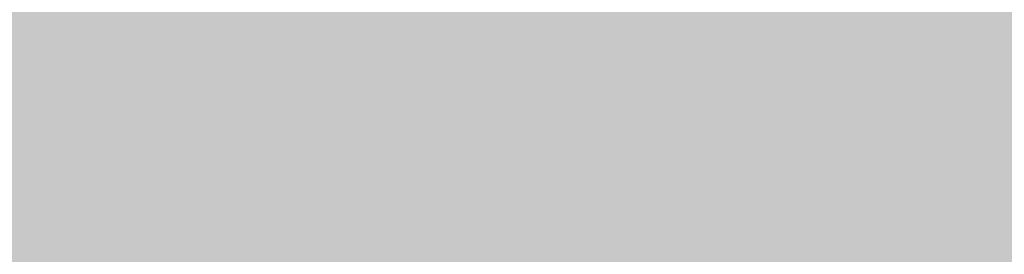
# Model space of a CAD drawing. Units: feet. Extents: x 3168 to 4724, y 827 to 1477.
# Tile 253 of 256: x 3384.42671 to 3384.48612, y 1099.00068 to 1099.01485. Entities that reach past the tile are written whole.
import ezdxf

# ---------------------------------------------------------------- set-up
doc = ezdxf.new("R2010")
doc.units = ezdxf.units.FT
doc.layers.add('A-ELEV', color=7, linetype='Continuous', lineweight=35)
doc.layers.add('A-ELEV-PATT', color=8, linetype='Continuous', lineweight=13)

msp = doc.modelspace()

# ---------------------------------------------------------------- hatches: boundary and pattern name
at = {"layer": 'A-ELEV-PATT'}
h = msp.add_hatch(color=256, dxfattribs=at)
h.dxf.hatch_style = 1
edge = h.paths.add_edge_path()
edge.add_ellipse((3552.905762, 979.220141), major_axis=(36.744924, 0), ratio=0.484848485, start_angle=0, end_angle=360)
edge = h.paths.add_edge_path()
edge.add_ellipse((3559.891637, 929.252282), major_axis=(36.744924, 0), ratio=0.484848485, start_angle=0, end_angle=360)
edge = h.paths.add_edge_path()
edge.add_line((3299.31681, 1198.606081), (3479.916714, 1198.606081))
edge.add_line((3479.916714, 1198.606081), (3479.916714, 1209.86857))
edge.add_spline(control_points=[(3479.916714, 1209.86857), (3464.301157, 1209.86857), (3448.685601, 1209.86857), (3410.949139, 1209.86857), (3388.828234, 1209.86857), (3355.646876, 1209.86857), (3344.586423, 1209.86857), (3327.995745, 1209.86857), (3322.465518, 1209.86857), (3314.170179, 1209.86857), (3311.405066, 1209.86857), (3307.257396, 1209.86857), (3305.874839, 1209.86857), (3303.801005, 1209.86857), (3303.109726, 1209.86857), (3302.072809, 1209.86857), (3301.72717, 1209.86857), (3301.208711, 1209.86857), (3301.035891, 1209.86857), (3300.776662, 1209.86857), (3300.690252, 1209.86857), (3300.560638, 1209.86857), (3300.517433, 1209.86857), (3300.452625, 1209.86857), (3300.431023, 1209.86857), (3300.398619, 1209.86857), (3300.387818, 1209.86857), (3300.366216, 1209.86857), (3300.345676, 1209.86857), (3300.345548, 1209.86857), (3300.345505, 1209.86857), (3300.343304, 1209.86857), (3300.341146, 1209.868571), (3300.337909, 1209.868571), (3300.33683, 1209.868572), (3300.333942, 1209.868573), (3300.332133, 1209.868574), (3300.325515, 1209.868577), (3300.320706, 1209.868581), (3300.310925, 1209.868592), (3300.305952, 1209.868598), (3300.290511, 1209.868623), (3300.280045, 1209.868646), (3300.232425, 1209.868777), (3300.195298, 1209.868954), (3299.951068, 1209.870608), (3299.744824, 1209.874326), (3299.436827, 1209.883257), (3299.334389, 1209.886792), (3299.181079, 1209.89292), (3299.130033, 1209.895099), (3298.652217, 1209.916801), (3298.22946, 1209.945718), (3297.601631, 1210.002367), (3297.393404, 1210.023464), (3297.082652, 1210.058309), (3296.979332, 1210.070458), (3296.292954, 1210.154861), (3295.718148, 1210.243356), (3294.868717, 1210.39885), (3294.5877, 1210.454478), (3294.169341, 1210.543349), (3294.030415, 1210.573878), (3291.707149, 1211.1012), (3289.65359, 1211.813435), (3285.776259, 1213.563988), (3283.95141, 1214.603478), (3280.512159, 1216.98008), (3278.897241, 1218.317592), (3276.379914, 1220.829489), (3275.416042, 1221.917738), (3274.039342, 1223.7077), (3273.581043, 1224.349535), (3273.143228, 1225.016316)], knot_values=[39.119033, 39.119033, 39.119033, 39.119033, 39.286353, 39.286353, 39.523379, 39.523379, 39.641892, 39.641892, 39.701148, 39.701148, 39.730777, 39.730777, 39.745591, 39.745591, 39.752998, 39.752998, 39.756701, 39.756701, 39.758553, 39.758553, 39.759479, 39.759479, 39.759942, 39.759942, 39.760173, 39.760173, 39.760289, 39.760289, 39.760405, 39.760405, 39.760463, 39.760463, 39.763389, 39.763389, 39.764851, 39.764851, 39.767304, 39.767304, 39.773825, 39.773825, 39.78057, 39.78057, 39.79477, 39.79477, 39.845194, 39.845194, 40.126715, 40.126715, 40.267476, 40.267476, 40.337856, 40.337856, 40.927023, 40.927023, 41.221606, 41.221606, 41.368898, 41.368898, 42.202622, 42.202622, 42.619485, 42.619485, 42.827916, 42.827916, 46.118323, 46.118323, 49.408731, 49.408731, 52.699139, 52.699139, 54.927489, 54.927489, 56.104228, 56.104228, 56.104228, 56.104228], weights=[1, 1, 1, 1, 1, 1, 1, 1, 1, 1, 1, 1, 1, 1, 1, 1, 1, 1, 1, 1, 1, 1, 1, 1, 1, 1, 1, 1, 1, 1, 1, 1, 1, 1, 1, 1, 1, 1, 1, 1, 1, 1, 1, 1, 1, 1, 1, 1, 1, 1, 1, 1, 1, 1, 1, 1, 1, 1, 1, 1, 1, 1, 1, 1, 1, 1, 1, 1, 1, 1, 1, 1, 1, 1], degree=3, periodic=0)
edge.add_line((3273.143228, 1225.016316), (3273.143228, 1099.016316))
edge.add_line((3273.143228, 1099.016316), (3299.31681, 1099.016316))
edge.add_line((3299.31681, 1099.016316), (3299.31681, 1198.606081))
edge = h.paths.add_edge_path()
edge.add_line((3304.758443, 1324.15806), (3479.916714, 1324.15806))
edge.add_line((3479.916714, 1324.15806), (3479.916714, 1335.714618))
edge.add_line((3479.916714, 1335.714618), (3269.161628, 1335.714618))
edge.add_spline(control_points=[(3269.161628, 1335.714618), (3264.024231, 1335.714618), (3258.364118, 1328.958189), (3259.264311, 1323.900274)], knot_values=[0, 0, 0, 0, 15.412191, 15.412191, 15.412191, 15.412191], degree=3, periodic=0)
edge.add_line((3259.264311, 1323.900274), (3265.516849, 1288.769135))
edge.add_line((3265.516849, 1288.769135), (3275.265103, 1261.545626))
edge.add_line((3275.265103, 1261.545626), (3304.758443, 1261.545626))
edge.add_line((3304.758443, 1261.545626), (3304.758443, 1324.15806))
h = msp.add_hatch(color=256, dxfattribs=at)
h.dxf.hatch_style = 1
h.paths.add_polyline_path([(3384.525247, 1099.016316), (3335.029168, 1099.016316), (3299.31681, 1099.016316), (3273.143228, 1099.016316), (3217.565364, 1099.016316), (3168.069285, 827.11626), (3335.029168, 827.11626)])

# ---------------------------------------------------------------- linework, layer by layer
at = {"layer": 'A-ELEV'}
msp.add_open_spline([(3808.5202, 1099.016316), (3808.5202, 1141.413235), (3808.5202, 1183.810154), (3808.5202, 1226.635324), (3808.5202, 1227.063576), (3808.5202, 1227.491828), (3811.491871, 1248.994673), (3814.463542, 1270.497518), (3817.46523, 1292.217564), (3817.495247, 1292.434764), (3817.525264, 1292.651964), (3817.572801, 1310.106748), (3817.620339, 1327.561532), (3817.667877, 1345.016316), (3817.667877, 1345.457962), (3817.667877, 1345.899608), (3817.667877, 1346.456047), (3817.667877, 1346.57084), (3817.667877, 1346.752887), (3817.667877, 1346.820142), (3817.667877, 1346.93487), (3817.667877, 1346.982345), (3817.667877, 1347.038587), (3817.667877, 1347.047356), (3817.667877, 1347.073661), (3817.667877, 1347.059303), (3817.667877, 1347.061545), (3817.667876, 1347.062667), (3817.667875, 1347.066031), (3817.667874, 1347.068274), (3817.66787, 1347.075001), (3817.667866, 1347.079486), (3817.667849, 1347.092937), (3817.667833, 1347.101902), (3817.667766, 1347.12879), (3817.667699, 1347.146705), (3817.667432, 1347.200421), (3817.667165, 1347.236192), (3817.6661, 1347.343385), (3817.665038, 1347.414686), (3817.660812, 1347.628095), (3817.656608, 1347.769708), (3817.63997, 1348.192487), (3817.623509, 1348.471586), (3817.559094, 1349.300067), (3817.496121, 1349.840588), (3817.255432, 1351.424156), (3817.026318, 1352.428785), (3816.306871, 1354.888914), (3815.743745, 1356.268727), (3814.463959, 1358.81921), (3813.746413, 1359.990968), (3812.195838, 1362.172343), (3811.362245, 1363.182124), (3809.588836, 1365.069009), (3808.648816, 1365.946105), (3806.654262, 1367.579616), (3805.599702, 1368.336154), (3803.352891, 1369.722327), (3802.160535, 1370.352386), (3799.600813, 1371.453586), (3798.232688, 1371.925481), (3795.280084, 1372.634624), (3793.693148, 1372.872068), (3791.869441, 1372.92648), (3791.740861, 1372.92922), (3791.353371, 1372.934101), (3791.092707, 1372.932901), (3790.304116, 1372.915068), (3789.769543, 1372.884195), (3789.20919, 1372.830236), (3789.190622, 1372.828424), (3789.134892, 1372.822912), (3789.097705, 1372.819137), (3789.048445, 1372.814008), (3789.0364, 1372.812743), (3789.000256, 1372.808918), (3788.976147, 1372.806325), (3788.949405, 1372.803404), (3788.946786, 1372.803118), (3788.942567, 1372.802655), (3788.940967, 1372.80248), (3788.938572, 1372.802217), (3788.937777, 1372.802129), (3788.935391, 1372.801867), (3788.867535, 1372.794402), (3788.756866, 1372.782228), (3788.701532, 1372.776141), (3788.53553, 1372.75788), (3788.424861, 1372.745707), (3788.092856, 1372.709185), (3787.871519, 1372.684837), (3787.207509, 1372.611793), (3786.764835, 1372.563097), (3785.436814, 1372.417009), (3784.551467, 1372.319617), (3781.895425, 1372.027442), (3780.12473, 1371.832658), (3774.812646, 1371.248307), (3771.271256, 1370.858739), (3760.647088, 1369.690037), (3753.56431, 1368.910902), (3732.315973, 1366.573498), (3718.150416, 1365.015228), (3694.006758, 1362.359326), (3684.028657, 1361.261694), (3674.050557, 1360.164062), (3664.600662, 1360.164062), (3655.150767, 1360.164062), (3626.801081, 1360.164062), (3607.901291, 1360.164062), (3551.20192, 1360.164062), (3513.40234, 1360.164062), (3467.725182, 1360.164062), (3459.847604, 1360.164062), (3436.214873, 1360.164062), (3420.459718, 1360.164062), (3373.194255, 1360.164062), (3341.683946, 1360.164062), (3302.848162, 1360.164062), (3295.522686, 1360.164062), (3286.038292, 1360.164062), (3283.879372, 1360.164062), (3277.402613, 1360.164062), (3273.084773, 1360.164062), (3267.732851, 1360.164062), (3266.698768, 1360.164062), (3263.59652, 1360.164062), (3261.528355, 1360.164062), (3259.236943, 1360.164062), (3259.013697, 1360.164062), (3258.343958, 1360.164062), (3257.897466, 1360.164062), (3257.430998, 1360.164062), (3257.411022, 1360.164062), (3257.370573, 1360.164062), (3257.37547, 1360.164062), (3257.374598, 1360.164062), (3257.373937, 1360.164062), (3257.371956, 1360.164062), (3257.370635, 1360.164061), (3257.366673, 1360.16406), (3257.364032, 1360.164059), (3257.356109, 1360.164053), (3257.350828, 1360.164047), (3257.334987, 1360.164023), (3257.32443, 1360.163998), (3257.292769, 1360.163899), (3257.271676, 1360.163799), (3257.208439, 1360.163398), (3257.166337, 1360.162995), (3257.040206, 1360.161388), (3256.956349, 1360.159783), (3256.705504, 1360.153393), (3256.53924, 1360.147036), (3256.04357, 1360.121916), (3255.717296, 1360.097102), (3254.752446, 1360.000481), (3254.127968, 1359.906513), (3252.180067, 1359.525332), (3250.941574, 1359.143991), (3248.670175, 1358.24329), (3247.635739, 1357.723834), (3245.732632, 1356.603471), (3244.863388, 1356.00206), (3243.253108, 1354.742865), (3242.511972, 1354.084731), (3240.751052, 1352.344781), (3239.800961, 1351.229574), (3238.087769, 1348.87244), (3237.324685, 1347.630355), (3235.98251, 1344.971632), (3235.402205, 1343.554907), (3234.591081, 1340.815458), (3234.310882, 1339.54355), (3233.97649, 1336.802561), (3233.922113, 1335.330877), (3234.148916, 1332.591269), (3234.349529, 1331.367201), (3234.719893, 1329.999367), (3234.752423, 1329.883362), (3234.853619, 1329.534797), (3234.925892, 1329.301685), (3235.024836, 1329.002552), (3235.046924, 1328.936928), (3235.077639, 1328.847239), (3235.085924, 1328.823198), (3235.110939, 1328.751064), (3235.127828, 1328.702962), (3235.147992, 1328.646242), (3235.151059, 1328.637632), (3235.156096, 1328.623526), (3235.158061, 1328.61803), (3235.160209, 1328.61203), (3235.165612, 1328.596943), (3235.180099, 1328.556486), (3235.190263, 1328.528101), (3235.220756, 1328.442946), (3235.241084, 1328.386176), (3235.302069, 1328.215865), (3235.342726, 1328.102325), (3235.464696, 1327.761704), (3235.54601, 1327.534623), (3235.78995, 1326.853381), (3235.952577, 1326.39922), (3236.440459, 1325.036736), (3236.765713, 1324.128414), (3237.741475, 1321.403446), (3238.391983, 1319.586801), (3240.343508, 1314.136866), (3241.644525, 1310.503576), (3245.547574, 1299.603706), (3248.149607, 1292.337126), (3255.955706, 1270.537385), (3261.159772, 1256.004225), (3267.387618, 1238.612001), (3268.411397, 1235.752937), (3269.510378, 1232.683864), (3269.585579, 1232.473854), (3269.706612, 1232.135851), (3269.752444, 1232.007857), (3269.827329, 1231.79873), (3269.856382, 1231.717595), (3269.906325, 1231.578122), (3269.927215, 1231.519782), (3269.972468, 1231.393406), (3269.996831, 1231.325368), (3270.026503, 1231.242506), (3270.031811, 1231.227681), (3270.040282, 1231.204024), (3270.039224, 1231.206979), (3270.039359, 1231.206601), (3270.039427, 1231.206412), (3270.03963, 1231.205846), (3270.039765, 1231.205468), (3270.040171, 1231.204335), (3270.040442, 1231.203579), (3270.041254, 1231.201313), (3270.041796, 1231.199802), (3270.04342, 1231.195269), (3270.044504, 1231.192248), (3270.047756, 1231.183185), (3270.049926, 1231.177145), (3270.056442, 1231.159028), (3270.060793, 1231.146957), (3270.073867, 1231.110761), (3270.082613, 1231.086656), (3270.108936, 1231.014413), (3270.1266, 1230.96635), (3270.179934, 1230.822457), (3270.215947, 1230.726923), (3270.325323, 1230.441508), (3270.400026, 1230.252811), (3270.629249, 1229.691444), (3270.788883, 1229.323501), (3271.286488, 1228.238319), (3271.6431, 1227.539755), (3272.775859, 1225.515277), (3273.614169, 1224.260502), (3275.416042, 1221.917738), (3276.379914, 1220.829489), (3278.897241, 1218.317592), (3280.512159, 1216.98008), (3283.95141, 1214.603478), (3285.776259, 1213.563988), (3289.65359, 1211.813435), (3291.707149, 1211.1012), (3294.030415, 1210.573878), (3294.169341, 1210.543349), (3294.5877, 1210.454478), (3294.868717, 1210.39885), (3295.718148, 1210.243356), (3296.292954, 1210.154861), (3296.979332, 1210.070458), (3297.082652, 1210.058309), (3297.393404, 1210.023464), (3297.601631, 1210.002367), (3298.22946, 1209.945718), (3298.652217, 1209.916801), (3299.130033, 1209.895099), (3299.181079, 1209.89292), (3299.334389, 1209.886792), (3299.436827, 1209.883257), (3299.744824, 1209.874326), (3299.951068, 1209.870608), (3300.195298, 1209.868954), (3300.232425, 1209.868777), (3300.280045, 1209.868646), (3300.290511, 1209.868623), (3300.305952, 1209.868598), (3300.310925, 1209.868592), (3300.320706, 1209.868581), (3300.325515, 1209.868577), (3300.332133, 1209.868574), (3300.333942, 1209.868573), (3300.33683, 1209.868572), (3300.337909, 1209.868571), (3300.341146, 1209.868571), (3300.343304, 1209.86857), (3300.345505, 1209.86857), (3300.345548, 1209.86857), (3300.345676, 1209.86857), (3300.366216, 1209.86857), (3300.387818, 1209.86857), (3300.398619, 1209.86857), (3300.431023, 1209.86857), (3300.452625, 1209.86857), (3300.517433, 1209.86857), (3300.560638, 1209.86857), (3300.690252, 1209.86857), (3300.776662, 1209.86857), (3301.035891, 1209.86857), (3301.208711, 1209.86857), (3301.72717, 1209.86857), (3302.072809, 1209.86857), (3303.109726, 1209.86857), (3303.801005, 1209.86857), (3305.874839, 1209.86857), (3307.257396, 1209.86857), (3311.405066, 1209.86857), (3314.170179, 1209.86857), (3322.465518, 1209.86857), (3327.995745, 1209.86857), (3344.586423, 1209.86857), (3355.646876, 1209.86857), (3388.828234, 1209.86857), (3410.949139, 1209.86857), (3477.311855, 1209.86857), (3521.553665, 1209.86857), (3566.836184, 1209.86857), (3567.876892, 1209.86857), (3570.999017, 1209.86857), (3573.080433, 1209.86857), (3575.781396, 1209.86857), (3576.400943, 1209.86857), (3577.295821, 1209.86857), (3577.571152, 1209.86857), (3578.397146, 1209.86857), (3578.947808, 1209.86857), (3579.756491, 1209.86857), (3580.014511, 1209.86857), (3580.342737, 1209.86857), (3580.326865, 1209.86857), (3580.32717, 1209.86857), (3580.327323, 1209.86857), (3580.327781, 1209.86857), (3580.328086, 1209.86857), (3580.329002, 1209.86857), (3580.329613, 1209.86857), (3580.331445, 1209.86857), (3580.332667, 1209.86857), (3580.336332, 1209.868569), (3580.338775, 1209.868567), (3580.346107, 1209.868563), (3580.350995, 1209.868558), (3580.365663, 1209.86854), (3580.375445, 1209.868522), (3580.404801, 1209.868449), (3580.424386, 1209.868376), (3580.483183, 1209.868085), (3580.522437, 1209.867793), (3580.640361, 1209.866624), (3580.719195, 1209.865454), (3580.956315, 1209.860766), (3581.115222, 1209.85607), (3581.594164, 1209.83723), (3581.916419, 1209.818331), (3582.889947, 1209.742428), (3583.547986, 1209.666169), (3585.531827, 1209.360617), (3586.867216, 1209.053886), (3589.471545, 1208.252472), (3590.740241, 1207.757852), (3591.995451, 1207.158802), (3592.057809, 1207.12874), (3592.244242, 1207.037954), (3592.367676, 1206.976632), (3592.73528, 1206.790359), (3592.976752, 1206.663101), (3593.244539, 1206.516441), (3593.274731, 1206.499825), (3593.365115, 1206.449839), (3593.425113, 1206.416333), (3593.604314, 1206.315285), (3593.722725, 1206.247211), (3593.857212, 1206.168398), (3593.874362, 1206.158319), (3593.925741, 1206.128041), (3593.959899, 1206.107798), (3594.062086, 1206.046899), (3594.129827, 1206.006074), (3594.208436, 1205.958171), (3594.219683, 1205.951304), (3594.253391, 1205.930686), (3594.275819, 1205.916917), (3594.342972, 1205.875536), (3594.387563, 1205.847853), (3594.433616, 1205.81905), (3594.435256, 1205.818024), (3594.440175, 1205.814946), (3594.443453, 1205.812894), (3594.447123, 1205.810594), (3594.447516, 1205.810348), (3594.448695, 1205.80961), (3594.449481, 1205.809117), (3594.450366, 1205.808562), (3594.450466, 1205.8085), (3594.4506, 1205.808415), (3594.467399, 1205.797887), (3594.493269, 1205.781674), (3594.506204, 1205.773568), (3594.545008, 1205.749248), (3594.570878, 1205.733035), (3594.648487, 1205.684396), (3594.700226, 1205.651969), (3594.855444, 1205.554691), (3594.958922, 1205.489839), (3595.269357, 1205.295282), (3595.476314, 1205.165577), (3596.097185, 1204.776463), (3596.511099, 1204.517054), (3597.752841, 1203.738826), (3598.580669, 1203.220007), (3601.064152, 1201.663551), (3602.719807, 1200.625914), (3607.686774, 1197.513002), (3610.998085, 1195.437727), (3620.932018, 1189.211903), (3627.55464, 1185.061354), (3647.422507, 1172.609707), (3660.667751, 1164.308608), (3700.403484, 1139.405313), (3726.893973, 1122.803116), (3757.205715, 1103.806052), (3761.02697, 1101.411184), (3764.848224, 1099.016316), (3745.328271, 1099.016316), (3725.808319, 1099.016316), (3706.288366, 1099.016316), (3706.288366, 1108.453237), (3706.288366, 1117.890158), (3706.288366, 1127.327079), (3710.750754, 1127.327079), (3715.213143, 1127.327079), (3719.675531, 1127.327079)], degree=3, knots=[0, 0, 0, 0, 0.982037, 0.982037, 0.991957, 0.991957, 0.991957, 1.966522, 1.966522, 1.976367, 1.976367, 1.976367, 2.976367, 2.976367, 2.976367, 3.00169, 3.00169, 3.008272, 3.008272, 3.012129, 3.012129, 3.014851, 3.014851, 3.015353, 3.015353, 3.016359, 3.016359, 3.017365, 3.017365, 3.019376, 3.019376, 3.023398, 3.023398, 3.031442, 3.031442, 3.047531, 3.047531, 3.079708, 3.079708, 3.144063, 3.144063, 3.272772, 3.272772, 3.53019, 3.53019, 4.045026, 4.045026, 5.074698, 5.074698, 6.700878, 6.700878, 8.327058, 8.327058, 9.953238, 9.953238, 11.579418, 11.579418, 13.205598, 13.205598, 14.831778, 14.831778, 16.457958, 16.457958, 18.084138, 18.084138, 18.206872, 18.206872, 18.45234, 18.45234, 18.943275, 18.943275, 18.960093, 18.960093, 18.993729, 18.993729, 19.00461, 19.00461, 19.026374, 19.026374, 19.028737, 19.028737, 19.03018, 19.03018, 19.030897, 19.030897, 19.032332, 19.032332, 19.033766, 19.033766, 19.036636, 19.036636, 19.042374, 19.042374, 19.053851, 19.053851, 19.076805, 19.076805, 19.122714, 19.122714, 19.21453, 19.21453, 19.398163, 19.398163, 19.765429, 19.765429, 20.024128, 20.024128, 20.024128, 20.092031, 20.092031, 20.227836, 20.227836, 20.499446, 20.499446, 20.556051, 20.556051, 20.66926, 20.66926, 20.895678, 20.895678, 20.948316, 20.948316, 20.963829, 20.963829, 20.994855, 20.994855, 21.002285, 21.002285, 21.017146, 21.017146, 21.01875, 21.01875, 21.021959, 21.021959, 21.022102, 21.022102, 21.022249, 21.022249, 21.022708, 21.022708, 21.023627, 21.023627, 21.025464, 21.025464, 21.029138, 21.029138, 21.036486, 21.036486, 21.051183, 21.051183, 21.080575, 21.080575, 21.139361, 21.139361, 21.256932, 21.256932, 21.492073, 21.492073, 21.962356, 21.962356, 23.01002, 23.01002, 24.057684, 24.057684, 25.105348, 25.105348, 26.153011, 26.153011, 27.776787, 27.776787, 29.400562, 29.400562, 31.024337, 31.024337, 32.278801, 32.278801, 33.533265, 33.533265, 34.467568, 34.467568, 34.553971, 34.553971, 34.726776, 34.726776, 34.775309, 34.775309, 34.793079, 34.793079, 34.82862, 34.82862, 34.834979, 34.834979, 34.839039, 34.839039, 34.839411, 34.839411, 34.840285, 34.840285, 34.842034, 34.842034, 34.845531, 34.845531, 34.852525, 34.852525, 34.866512, 34.866512, 34.894488, 34.894488, 34.950439, 34.950439, 35.062342, 35.062342, 35.286147, 35.286147, 35.733758, 35.733758, 35.821815, 35.821815, 35.828283, 35.828283, 35.832225, 35.832225, 35.834724, 35.834724, 35.836521, 35.836521, 35.838617, 35.838617, 35.839073, 35.839073, 35.839345, 35.839345, 35.839617, 35.839617, 35.840161, 35.840161, 35.841249, 35.841249, 35.843425, 35.843425, 35.847778, 35.847778, 35.856482, 35.856482, 35.873891, 35.873891, 35.908709, 35.908709, 35.978345, 35.978345, 36.117617, 36.117617, 36.396161, 36.396161, 36.953248, 36.953248, 38.067423, 38.067423, 40.295772, 40.295772, 42.524122, 42.524122, 45.81453, 45.81453, 49.104937, 49.104937, 52.395345, 52.395345, 52.603776, 52.603776, 53.020639, 53.020639, 53.854363, 53.854363, 54.001655, 54.001655, 54.296238, 54.296238, 54.885405, 54.885405, 54.955785, 54.955785, 55.096546, 55.096546, 55.378067, 55.378067, 55.42849, 55.42849, 55.442691, 55.442691, 55.449436, 55.449436, 55.455957, 55.455957, 55.458409, 55.458409, 55.459872, 55.459872, 55.462798, 55.462798, 55.462856, 55.462856, 55.462972, 55.462972, 55.463088, 55.463088, 55.463319, 55.463319, 55.463782, 55.463782, 55.464708, 55.464708, 55.46656, 55.46656, 55.470263, 55.470263, 55.47767, 55.47767, 55.492484, 55.492484, 55.522112, 55.522112, 55.581369, 55.581369, 55.699882, 55.699882, 55.936907, 55.936907, 56.410959, 56.410959, 56.42211, 56.42211, 56.444413, 56.444413, 56.451051, 56.451051, 56.454001, 56.454001, 56.459901, 56.459901, 56.462666, 56.462666, 56.463418, 56.463418, 56.464171, 56.464171, 56.465675, 56.465675, 56.468684, 56.468684, 56.474702, 56.474702, 56.486738, 56.486738, 56.51081, 56.51081, 56.558955, 56.558955, 56.655243, 56.655243, 56.847821, 56.847821, 57.232975, 57.232975, 58.003284, 58.003284, 59.543901, 59.543901, 62.625137, 62.625137, 68.787607, 68.787607, 74.950078, 74.950078, 75.27336, 75.27336, 75.919923, 75.919923, 77.213051, 77.213051, 77.377769, 77.377769, 77.707206, 77.707206, 78.366079, 78.366079, 78.462532, 78.462532, 78.655436, 78.655436, 79.041245, 79.041245, 79.105735, 79.105735, 79.234714, 79.234714, 79.492672, 79.492672, 79.502197, 79.502197, 79.521249, 79.521249, 79.523534, 79.523534, 79.528103, 79.528103, 79.528682, 79.528682, 79.528885, 79.528885, 79.529089, 79.529089, 79.529495, 79.529495, 79.530308, 79.530308, 79.531935, 79.531935, 79.535187, 79.535187, 79.541693, 79.541693, 79.554704, 79.554704, 79.580725, 79.580725, 79.632769, 79.632769, 79.736856, 79.736856, 79.94503, 79.94503, 80.361377, 80.361377, 80.421435, 80.421435, 80.421435, 81.421435, 81.421435, 81.421435, 82.421435, 82.421435, 82.421435, 83.421435, 83.421435, 83.421435, 83.421435], dxfattribs=at)

doc.saveas('drawing.dxf')
